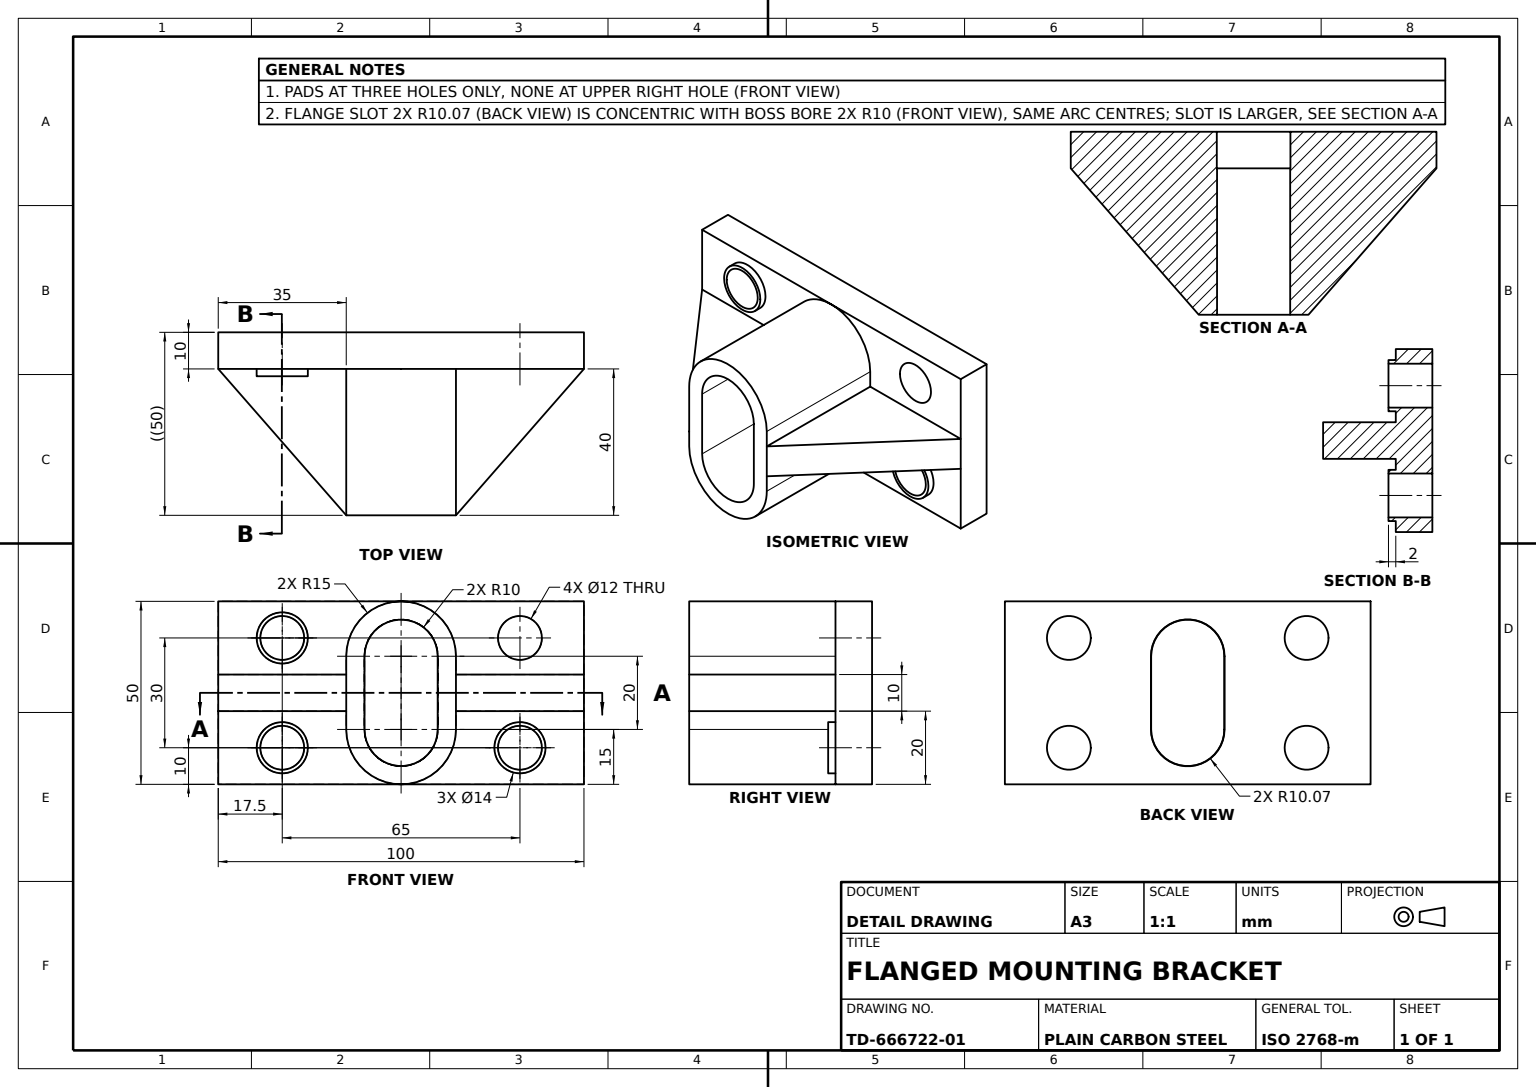
SolidWorks part; units mm, degrees
material "Plain Carbon Steel"
ref_plane "Front Plane" through (0, 0, 0) normal (0, 0, 1) x (1, 0, 0)
ref_plane "Top Plane" through (0, 0, 0) normal (0, 1, 0) x (1, 0, 0)
ref_plane "Right Plane" through (0, 0, 0) normal (1, 0, 0) x (0, 0, -1)
sketch "Base Plate Sketch" plane through (0, 0, 0) normal (0, 0, 1) x (1, 0, 0)
  line L0 (0, 0) -> (100, 0)
  line L1 (100, 0) -> (100, 50)
  line L2 (100, 50) -> (0, 50)
  line L3 (0, 50) -> (0, 0)
  dimension "D1" = 100
  dimension "D2" = 50
extrude "Base Plate 100x50x10" add sketch "Base Plate Sketch" along normal blind 10
sketch "Oval Boss Sketch" plane through (0, 0, 10) normal (0, 0, 1) x (1, 0, 0)
  line L0 (50, 15) -> (50, 35) construction
  line L1 (0, 50) -> (0, 0) construction
  line L2 (40, 15) -> (40, 35)
  line L3 (60, 15) -> (60, 35)
  line L4 (100, 50) -> (0, 50) construction
  line L5 (50, 15) -> (50, 35) construction
  line L6 (35, 15) -> (35, 35)
  line L7 (65, 15) -> (65, 35)
  arc A0 (40, 15) -> (60, 15) centre (50, 15) ccw
  arc A1 (60, 35) -> (40, 35) centre (50, 35) ccw
  arc A2 (35, 15) -> (65, 15) centre (50, 15) ccw
  arc A3 (65, 35) -> (35, 35) centre (50, 35) ccw
  point P4 (50, 25)
  point P10 (0, 25)
  point P13 (50, 50)
  point P14 (50, 25)
  dimension "D1" = 10
  dimension "D3" = 15
  dimension "D2" = 20
extrude "Oval Boss" add sketch "Oval Boss Sketch" along normal blind 40
ref_plane "Plane1" through (0, 25, 0) normal (0, 1, 0) x (1, 0, 0)
sketch "Support Rib 1 Sketch" plane through (0, 25, 0) normal (0, 1, 0) x (1, 0, 0)
  line L0 (65, -50) -> (100, -10)
rib "Support Rib 1" sketch "Support Rib 1 Sketch" sketch "Support Rib 1 Sketch" thickness 10 extrusion direction parallel to sketch draft on no parameters "D1"=10
sketch "Support Rib 2 Sketch" plane through (0, 25, 0) normal (0, 1, 0) x (1, 0, 0)
  line L0 (35, -50) -> (0, -10)
rib "Support Rib 2" sketch "Support Rib 2 Sketch" sketch "Support Rib 2 Sketch" thickness 10 extrusion direction parallel to sketch draft on no parameters "D1"=10
sketch "Raised Pads Sketch" plane through (0, 0, 10) normal (0, 0, 1) x (1, 0, 0)
  line L0 (0, 0) -> (17.5, 0) construction
  line L1 (0, 0) -> (50, 0) construction
  line L2 (17.5, 0) -> (17.5, 10) construction
  line L3 (100, 0) -> (82.5, 0) construction
  line L4 (50, 0) -> (100, 0) construction
  line L5 (82.5, 0) -> (82.5, 10) construction
  line L6 (0, 20) -> (0, 0) construction
  line L7 (35, 20) -> (0, 20) construction
  line L9 (100, 50) -> (82.5, 50) construction
  line L10 (100, 50) -> (50, 50) construction
  line L11 (82.5, 50) -> (82.5, 40) construction
  circle A0 centre (17.5, 10) radius 6
  circle A1 centre (17.5, 10) radius 7
  circle A2 centre (82.5, 10) radius 6
  circle A3 centre (82.5, 10) radius 7
  circle A4 centre (17.5, 40) radius 6
  circle A5 centre (17.5, 40) radius 7
  circle A6 centre (82.5, 40) radius 6
  dimension "D1" = 12
  dimension "D2" = 14
  dimension "D3" = 12
  dimension "D4" = 14
  dimension "D5" = 12
  dimension "D6" = 14
  dimension "D7" = 17.5
  dimension "D8" = 20
extrude "Raised Pads 2mm" add sketch "Raised Pads Sketch" along normal blind 2
sketch "Mounting Hole 1 Sketch" plane through (0, 0, 10) normal (0, 0, 1) x (1, 0, 0)
  circle A0 centre (17.5, 40) radius 6
  dimension "D1" = 12
extrude "Mounting Hole 1" cut sketch "Mounting Hole 1 Sketch" against normal through all
sketch "Mounting Hole 2 Sketch" plane through (0, 0, 10) normal (0, 0, 1) x (1, 0, 0)
  circle A0 centre (17.5, 10) radius 6
  dimension "D1" = 12
extrude "Mounting Hole 2" cut sketch "Mounting Hole 2 Sketch" against normal through all
sketch "Mounting Hole 3 Sketch" plane through (0, 0, 12) normal (0, 0, 1) x (1, 0, 0)
  circle A0 centre (82.5, 40) radius 6
  dimension "D1" = 12
extrude "Mounting Hole 3" cut sketch "Mounting Hole 3 Sketch" against normal through all
sketch "Mounting Hole 4 Sketch" plane through (0, 0, 10) normal (0, 0, 1) x (1, 0, 0)
  circle A0 centre (82.5, 10) radius 6
  dimension "D1" = 12
extrude "Mounting Hole 4" cut sketch "Mounting Hole 4 Sketch" against normal through all
sketch "Boss Bore Sketch" plane through (0, 0, 10) normal (0, 0, 1) x (1, 0, 0)
  line L0 (50, 15) -> (50, 35) construction
  line L1 (39.9346, 15) -> (39.9346, 35)
  line L2 (60.0654, 15) -> (60.0654, 35)
  arc A0 (39.9346, 15) -> (60.0654, 15) centre (50, 15) ccw
  arc A1 (60.0654, 35) -> (39.9346, 35) centre (50, 35) ccw
  point P2 (50, 25)
  dimension "D1" = 10.0654
extrude "Boss Bore" cut sketch "Boss Bore Sketch" against normal through all
